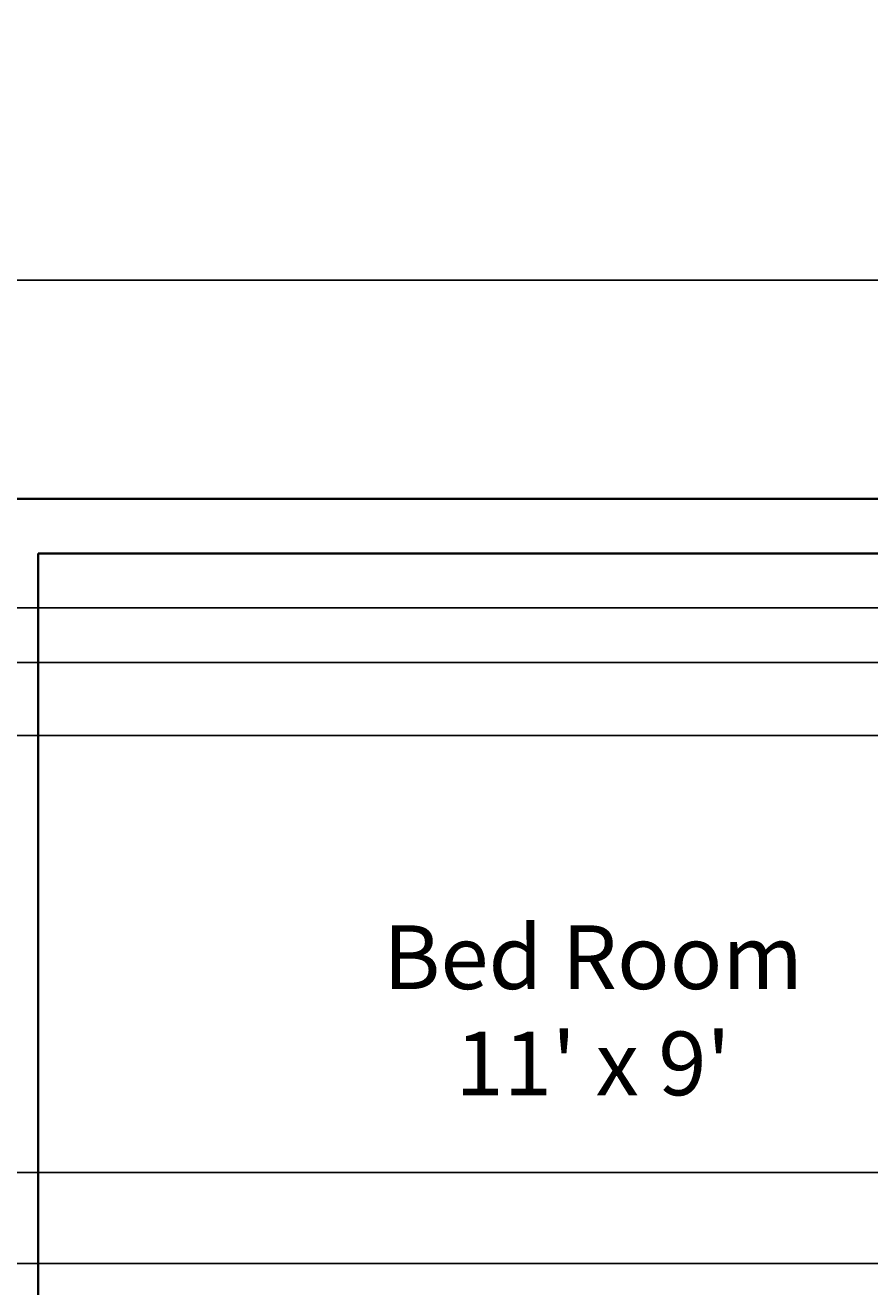
# Model space of a CAD drawing. Units: feet. Extents: x 105 to 1094, y -88 to 588.
# Tile 4 of 59: x 155 to 248, y 138 to 276. Entities that reach past the tile are written whole.
import ezdxf

# ---------------------------------------------------------------- set-up
doc = ezdxf.new("R2010")
doc.units = ezdxf.units.FT
doc.header["$MEASUREMENT"] = 0
for name, color, linetype, lineweight in [('A-ANNO-DIMS', 2, 'Continuous', 18), ('A-AREA-IDEN', 7, 'Continuous', 18), ('A-WALL', 7, 'Continuous', 35)]:
    doc.layers.add(name, color=color, linetype=linetype, lineweight=lineweight)
doc.styles.get("Standard").update_dxf_attribs({"font": 'arial.ttf'})
doc.dimstyles.get("Standard").update_dxf_attribs({"dimtxt": 0.18, "dimasz": 0.18, "dimexe": 0.18, "dimexo": 0.0625, "dimgap": 0.09, "dimtad": 0, "dimtih": 1, "dimtoh": 1, "dimdec": 4, "dimzin": 0, "dimdsep": 46, "dimtxsty": 'Standard', "dimcen": 0.09, "dimadec": 0, "dimazin": 0, "dimtfac": 1, "dimtdec": 4, "dimtofl": 0, "dimtmove": 0, "dimatfit": 3, "dimfxl": 1, "dimtolj": 1, "dimtzin": 0, "dimarcsym": 0})

# ---------------------------------------------------------------- blocks, each defined once
blk = doc.blocks.new('*D20')
at = {"layer": 'A-ANNO-DIMS', "color": 0, "lineweight": -2, "transparency": 16777216}
for p, q in [((150.69, 276.02), (150.69, -88.15)), ((1048.69, 276.02), (1048.69, -88.15)), ((150.87, -87.97), (599.4, -87.97)), ((1048.51, -87.97), (599.98, -87.97))]:
    blk.add_line(p, q, dxfattribs=at)
at = {"layer": 'A-ANNO-DIMS', "color": 0, "transparency": 16777216}
for points in [[(150.87, -87.94), (150.87, -88), (150.69, -87.97)], [(1048.51, -87.94), (1048.51, -88), (1048.69, -87.97)]]:
    blk.add_solid(points, dxfattribs=at)
at = {"layer": 'Defpoints', "color": 0, "transparency": 16777216}
for p in [(150.69, 276.08), (1048.69, 276.08), (1048.69, -87.97)]:
    blk.add_point(p, dxfattribs=at)
at = {"layer": 'A-ANNO-DIMS', "color": 0, "transparency": 16777216, "insert": (599.69, -87.97), "char_height": 0.18, "attachment_point": 5}
blk.add_mtext('\\A1;898', dxfattribs=at)
blk = doc.blocks.new('*D21')
at = {"layer": 'A-ANNO-DIMS', "color": 0, "lineweight": -2, "transparency": 16777216}
for p, q in [((849.63, 543.08), (105.46, 543.08)), ((105.64, 542.9), (105.64, 250.26)), ((105.64, -42.74), (105.64, 249.9)), ((849.63, -42.92), (105.46, -42.92))]:
    blk.add_line(p, q, dxfattribs=at)
at = {"layer": 'A-ANNO-DIMS', "color": 0, "transparency": 16777216}
for points in [[(105.61, 542.9), (105.67, 542.9), (105.64, 543.08)], [(105.61, -42.74), (105.67, -42.74), (105.64, -42.92)]]:
    blk.add_solid(points, dxfattribs=at)
at = {"layer": 'Defpoints', "color": 0, "transparency": 16777216}
for p in [(105.64, 543.08), (849.69, 543.08), (849.69, -42.92)]:
    blk.add_point(p, dxfattribs=at)
at = {"layer": 'A-ANNO-DIMS', "color": 0, "transparency": 16777216, "insert": (105.64, 250.08), "char_height": 0.18, "attachment_point": 5}
blk.add_mtext('\\A1;586', dxfattribs=at)
blk = doc.blocks.new('*D36')
at = {"layer": 'A-ANNO-DIMS', "color": 0, "lineweight": -2, "transparency": 16777216}
for p, q in [((547.24, 248.08), (105.46, 248.08)), ((105.64, 247.9), (105.64, 230.26)), ((105.64, 212.26), (105.64, 229.9)), ((546.63, 212.08), (105.46, 212.08))]:
    blk.add_line(p, q, dxfattribs=at)
at = {"layer": 'A-ANNO-DIMS', "color": 0, "transparency": 16777216}
for points in [[(105.61, 247.9), (105.67, 247.9), (105.64, 248.08)], [(105.61, 212.26), (105.67, 212.26), (105.64, 212.08)]]:
    blk.add_solid(points, dxfattribs=at)
at = {"layer": 'Defpoints', "color": 0, "transparency": 16777216}
for p in [(105.64, 248.08), (547.3, 248.08), (546.69, 212.08)]:
    blk.add_point(p, dxfattribs=at)
at = {"layer": 'A-ANNO-DIMS', "color": 0, "transparency": 16777216, "insert": (105.64, 230.08), "char_height": 0.18, "attachment_point": 5}
blk.add_mtext('\\A1;36', dxfattribs=at)
blk = doc.blocks.new('*D38')
at = {"layer": 'A-ANNO-DIMS', "color": 0, "lineweight": -2, "transparency": 16777216}
for p, q in [((150.69, 224.14), (150.69, 588.31)), ((150.87, 588.13), (222.41, 588.13)), ((294.51, 588.13), (222.97, 588.13)), ((294.69, 224.14), (294.69, 588.31))]:
    blk.add_line(p, q, dxfattribs=at)
at = {"layer": 'A-ANNO-DIMS', "color": 0, "transparency": 16777216}
for points in [[(150.87, 588.16), (150.87, 588.1), (150.69, 588.13)], [(294.51, 588.16), (294.51, 588.1), (294.69, 588.13)]]:
    blk.add_solid(points, dxfattribs=at)
at = {"layer": 'Defpoints', "color": 0, "transparency": 16777216}
for p in [(294.69, 588.13), (150.69, 224.08), (294.69, 224.08)]:
    blk.add_point(p, dxfattribs=at)
at = {"layer": 'A-ANNO-DIMS', "color": 0, "transparency": 16777216, "insert": (222.69, 588.13), "char_height": 0.18, "attachment_point": 5}
blk.add_mtext('\\A1;144', dxfattribs=at)
blk = doc.blocks.new('*D46')
at = {"layer": 'A-ANNO-DIMS', "color": 0, "lineweight": -2, "transparency": 16777216}
for p, q in [((580.63, 206.08), (105.46, 206.08)), ((105.64, 205.9), (105.64, 173.26)), ((105.64, 140.26), (105.64, 172.9)), ((580.63, 140.08), (105.46, 140.08))]:
    blk.add_line(p, q, dxfattribs=at)
at = {"layer": 'A-ANNO-DIMS', "color": 0, "transparency": 16777216}
for points in [[(105.61, 205.9), (105.67, 205.9), (105.64, 206.08)], [(105.61, 140.26), (105.67, 140.26), (105.64, 140.08)]]:
    blk.add_solid(points, dxfattribs=at)
at = {"layer": 'Defpoints', "color": 0, "transparency": 16777216}
for p in [(580.69, 206.08), (105.64, 140.08), (580.69, 140.08)]:
    blk.add_point(p, dxfattribs=at)
at = {"layer": 'A-ANNO-DIMS', "color": 0, "transparency": 16777216, "insert": (105.64, 173.08), "char_height": 0.18, "attachment_point": 5}
blk.add_mtext('\\A1;66', dxfattribs=at)
blk = doc.blocks.new('*D55')
at = {"layer": 'A-ANNO-DIMS', "color": 0, "lineweight": -2, "transparency": 16777216}
for p, q in [((292.63, 198.08), (105.46, 198.08)), ((105.64, 197.9), (105.64, 174.26)), ((105.64, 150.26), (105.64, 173.9)), ((293.13, 150.08), (105.46, 150.08))]:
    blk.add_line(p, q, dxfattribs=at)
at = {"layer": 'A-ANNO-DIMS', "color": 0, "transparency": 16777216}
for points in [[(105.61, 197.9), (105.67, 197.9), (105.64, 198.08)], [(105.61, 150.26), (105.67, 150.26), (105.64, 150.08)]]:
    blk.add_solid(points, dxfattribs=at)
at = {"layer": 'Defpoints', "color": 0, "transparency": 16777216}
for p in [(105.64, 198.08), (292.69, 198.08), (293.2, 150.08)]:
    blk.add_point(p, dxfattribs=at)
at = {"layer": 'A-ANNO-DIMS', "color": 0, "transparency": 16777216, "insert": (105.64, 174.08), "char_height": 0.18, "attachment_point": 5}
blk.add_mtext('\\A1;48', dxfattribs=at)

msp = doc.modelspace()

# ---------------------------------------------------------------- linework, layer by layer
at = {"layer": 'A-WALL'}
for p, q in [((294.6883, 224.0812), (150.6883, 224.0812)), ((288.6883, 218.0812), (156.6883, 218.0812)), ((156.6883, 218.0812), (156.6883, 110.0812))]:
    msp.add_line(p, q, dxfattribs=at)

# ---------------------------------------------------------------- texts
at = {"layer": 'A-AREA-IDEN', "insert": (266.8257, 158.5586), "char_height": 7, "attachment_point": 9}
msp.add_mtext_dynamic_manual_height_columns("\\pxqc;Bed Room \\P11' x 9'", width=98.34246, gutter_width=1, heights=[0], dxfattribs=at)

# ---------------------------------------------------------------- dimensions: what is measured, and where the dimension line sits
at = {"layer": 'A-ANNO-DIMS'}
for base, p1, p2, picture, middle in [((294.6883, 588.1312), (150.6883, 224.0812), (294.6883, 224.0812), '*D38', (222.6883, 588.1312)), ((1048.6883, -87.9688), (150.6883, 276.0812), (1048.6883, 276.0812), '*D20', (599.6883, -87.9688))]:
    dim = msp.add_linear_dim(base=base, p1=p1, p2=p2, dimstyle='Standard', override={"dimdec": 0, "dimlfac": 1, "dimrnd": 0, "dimzin": 0, "dimdsep": 46, "dimlunit": 2}, dxfattribs=at)
    dim.commit()
    dim.dimension.update_dxf_attribs({"geometry": picture, "text_midpoint": middle})
for base, p1, p2, picture, middle in [((105.6383, 543.0812), (849.6883, -42.9188), (849.6883, 543.0812), '*D21', (105.6383, 250.0812)), ((105.6383, 248.0812), (546.6883, 212.0812), (547.2975, 248.0812), '*D36', (105.6383, 230.0812)), ((105.6383, 140.0812), (580.6883, 206.0812), (580.6883, 140.0812), '*D46', (105.6383, 173.0812)), ((105.6383, 198.0812), (293.1967, 150.0812), (292.6883, 198.0812), '*D55', (105.6383, 174.0812))]:
    dim = msp.add_linear_dim(base=base, p1=p1, p2=p2, angle=90, dimstyle='Standard', override={"dimdec": 0, "dimlfac": 1, "dimrnd": 0, "dimzin": 0, "dimdsep": 46, "dimlunit": 2}, dxfattribs=at)
    dim.commit()
    dim.dimension.update_dxf_attribs({"geometry": picture, "text_midpoint": middle})

doc.saveas('drawing.dxf')
